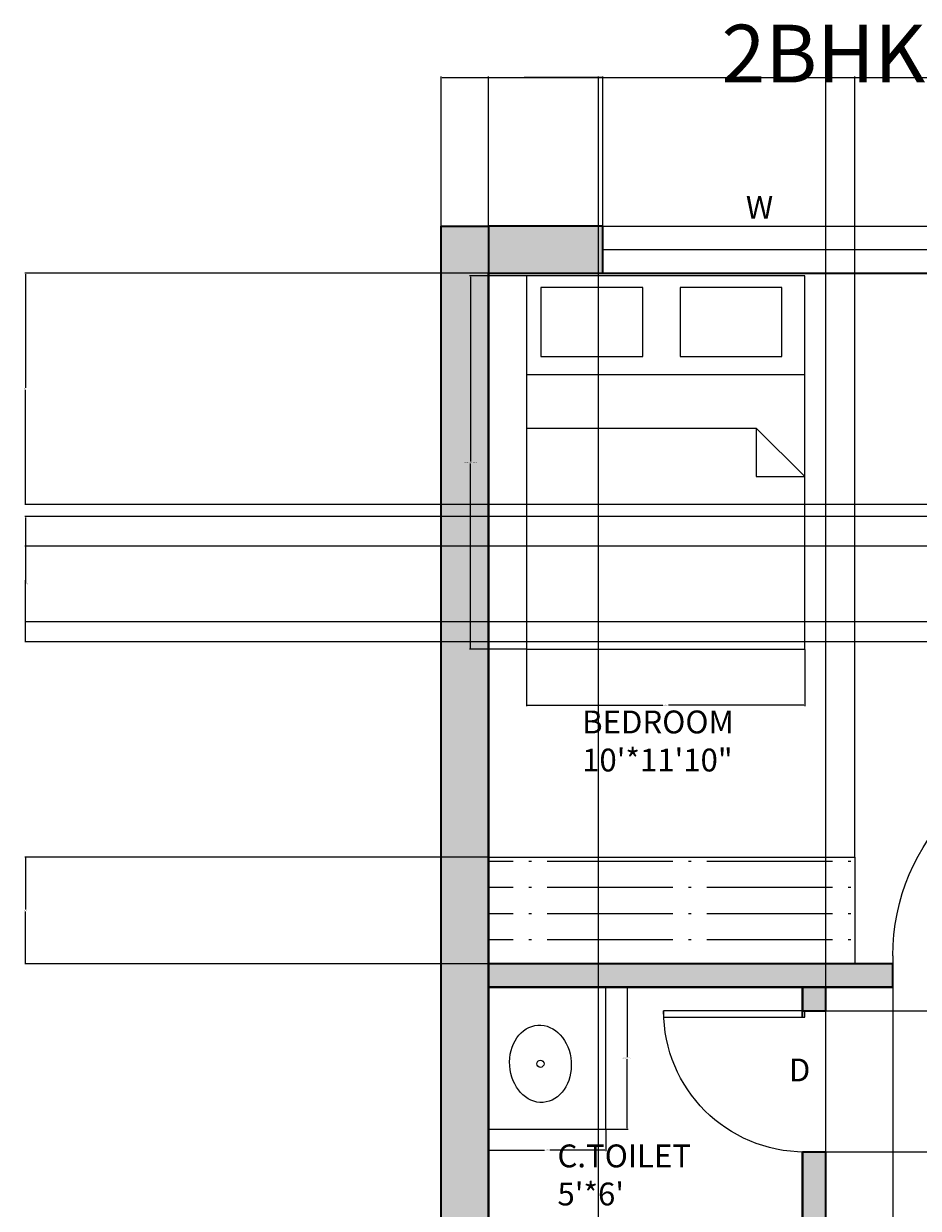
# Model space of a CAD drawing. Units: inches. Extents: x 2035 to 2384, y 1427 to 2020.
# Tile 5 of 7: x 2035 to 2206, y 1794 to 2020. Entities that reach past the tile are written whole.
import ezdxf

# ---------------------------------------------------------------- set-up
doc = ezdxf.new("R2010")
doc.units = ezdxf.units.IN
for name, color, linetype, lineweight in [('A-ANNO-DIMS', 2, 'Continuous', 18), ('A-ANNO-IDEN', 201, 'Continuous', 18), ('A-ANNO-TITL', 7, 'Continuous', 35), ('A-AREA-IDEN', 201, 'Continuous', 18), ('A-FLOR-CABN', 71, 'Continuous', 18), ('A-FLOR-CABN-PATT', 71, 'Continuous', 13), ('A-FLOR-FIXT', 9, 'Continuous', 18), ('A-WALL-PATT', 140, 'Continuous', 13), ('C-PROP', 7, 'Continuous', 25), ('DOOR', 52, 'Continuous', 25), ('FUR', 71, 'Continuous', 18), ('WALL', 140, 'Continuous', 35), ('WIN', 230, 'Continuous', 18)]:
    doc.layers.add(name, color=color, linetype=linetype, lineweight=lineweight)
doc.styles.get("Standard").update_dxf_attribs({"font": 'arial.ttf'})
doc.dimstyles.get("Standard").update_dxf_attribs({"dimtxt": 0.18, "dimasz": 0.18, "dimexe": 0.18, "dimexo": 0.0625, "dimgap": 0.09, "dimtad": 0, "dimtih": 1, "dimtoh": 1, "dimdec": 4, "dimzin": 0, "dimdsep": 46, "dimtxsty": 'Standard', "dimcen": 0.09, "dimadec": 0, "dimazin": 0, "dimtfac": 1, "dimtdec": 4, "dimtofl": 0, "dimtmove": 0, "dimatfit": 3, "dimfxl": 1, "dimtolj": 1, "dimtzin": 0, "dimarcsym": 0})

# ---------------------------------------------------------------- blocks, each defined once
blk = doc.blocks.new('*U2')
for p, q in [((0, 0), (0, -6)), ((40, 0), (40, -6))]:
    blk.add_line(p, q)
blk.add_lwpolyline([(0, 0), (0, 40), (1.75, 40), (1.75, 0)], close=True)
blk.add_arc((0, 0), 40, 0, 90)
blk = doc.blocks.new('BED-DOUBLE')
for p, q in [((18.86, 0), (18.86, 53.15)), ((38.37, 53.15), (29.1, 43.9)), ((38.37, 43.9), (38.37, 53.15)), ((29.1, 0), (29.1, 43.9)), ((29.1, 43.9), (38.37, 43.9))]:
    blk.add_line(p, q)
for points in [[(0, 0), (71.34, 0), (71.34, 53.15), (0, 53.15)], [(2.2, 29.34), (15.42, 29.34), (15.42, 48.81), (2.2, 48.81)], [(2.2, 2.74), (15.42, 2.74), (15.42, 22.21), (2.2, 22.21)]]:
    blk.add_lwpolyline(points, close=True)
blk = doc.blocks.new('BASIN-VANITY')
blk.add_lwpolyline([(0, 0), (22.45, 0), (22.45, 27.1), (0, 27.1)], close=True)
blk.add_circle((9.95, 12.48), 0.683)
blk.add_ellipse((9.95, 12.48), major_axis=(-0.5, 7.38), ratio=0.795414)
blk = doc.blocks.new('WIN-BEDROOM')
blk.add_line((0, 4.5), (63.76, 4.5))
blk.add_lwpolyline([(0, 9), (63.76, 9), (63.76, 0), (0, 0)], close=True)
blk = doc.blocks.new('*D12')
at = {"layer": 'A-ANNO-DIMS', "color": 0, "lineweight": -2, "transparency": 16777216}
for p, q in [((2130.97, 1971.85), (2120.15, 1971.85)), ((2120.33, 1971.67), (2120.33, 1936.36)), ((2120.33, 1900.69), (2120.33, 1935.99)), ((2130.97, 1900.51), (2120.15, 1900.51))]:
    blk.add_line(p, q, dxfattribs=at)
at = {"layer": 'A-ANNO-DIMS', "color": 0, "lineweight": 100, "transparency": 16777216}
for points in [[(2120.3, 1971.67), (2120.36, 1971.67), (2120.33, 1971.85)], [(2120.3, 1900.69), (2120.36, 1900.69), (2120.33, 1900.51)]]:
    blk.add_solid(points, dxfattribs=at)
at = {"layer": 'Defpoints', "color": 0, "lineweight": 100, "transparency": 16777216}
for p in [(2131.03, 1971.85), (2120.33, 1900.51), (2131.03, 1900.51)]:
    blk.add_point(p, dxfattribs=at)
at = {"layer": 'A-ANNO-DIMS', "color": 0, "transparency": 16777216, "insert": (2120.33, 1936.18), "char_height": 0.18, "attachment_point": 5}
blk.add_mtext('\\A1;DOUBLE BED 71 TYP.', dxfattribs=at)
blk = doc.blocks.new('*D13')
at = {"layer": 'A-ANNO-DIMS', "color": 0, "lineweight": -2, "transparency": 16777216}
for p, q in [((2131.03, 1900.45), (2131.03, 1889.63)), ((2184.19, 1900.45), (2184.19, 1889.63)), ((2131.21, 1889.81), (2157.08, 1889.81)), ((2184.01, 1889.81), (2158.14, 1889.81))]:
    blk.add_line(p, q, dxfattribs=at)
at = {"layer": 'A-ANNO-DIMS', "color": 0, "lineweight": 100, "transparency": 16777216}
for points in [[(2131.21, 1889.84), (2131.21, 1889.78), (2131.03, 1889.81)], [(2184.01, 1889.84), (2184.01, 1889.78), (2184.19, 1889.81)]]:
    blk.add_solid(points, dxfattribs=at)
at = {"layer": 'Defpoints', "color": 0, "lineweight": 100, "transparency": 16777216}
for p in [(2131.03, 1900.51), (2184.19, 1900.51), (2184.19, 1889.81)]:
    blk.add_point(p, dxfattribs=at)
at = {"layer": 'A-ANNO-DIMS', "color": 0, "transparency": 16777216, "insert": (2157.61, 1889.81), "char_height": 0.18, "attachment_point": 5}
blk.add_mtext('\\A1;53 TYP.', dxfattribs=at)
blk = doc.blocks.new('*D18')
at = {"layer": 'A-ANNO-DIMS', "color": 0, "lineweight": -2, "transparency": 16777216}
for p, q in [((2146.26, 1835.88), (2150.44, 1835.88)), ((2150.26, 1835.7), (2150.26, 1822.51)), ((2150.26, 1808.96), (2150.26, 1822.15)), ((2146.26, 1808.78), (2150.44, 1808.78))]:
    blk.add_line(p, q, dxfattribs=at)
at = {"layer": 'A-ANNO-DIMS', "color": 0, "lineweight": 100, "transparency": 16777216}
for points in [[(2150.23, 1835.7), (2150.29, 1835.7), (2150.26, 1835.88)], [(2150.23, 1808.96), (2150.29, 1808.96), (2150.26, 1808.78)]]:
    blk.add_solid(points, dxfattribs=at)
at = {"layer": 'Defpoints', "color": 0, "lineweight": 100, "transparency": 16777216}
for p in [(2146.2, 1835.88), (2150.26, 1835.88), (2146.2, 1808.78)]:
    blk.add_point(p, dxfattribs=at)
at = {"layer": 'A-ANNO-DIMS', "color": 0, "transparency": 16777216, "insert": (2150.26, 1822.33), "char_height": 0.18, "attachment_point": 5}
blk.add_mtext('\\A1;VANITY 27 TYP.', dxfattribs=at)
blk = doc.blocks.new('*D19')
at = {"layer": 'A-ANNO-DIMS', "color": 0, "lineweight": -2, "transparency": 16777216}
for p, q in [((2123.75, 1808.72), (2123.75, 1804.54)), ((2146.2, 1808.72), (2146.2, 1804.54)), ((2123.93, 1804.72), (2134.45, 1804.72)), ((2146.02, 1804.72), (2135.51, 1804.72))]:
    blk.add_line(p, q, dxfattribs=at)
at = {"layer": 'A-ANNO-DIMS', "color": 0, "lineweight": 100, "transparency": 16777216}
for points in [[(2123.93, 1804.75), (2123.93, 1804.69), (2123.75, 1804.72)], [(2146.02, 1804.75), (2146.02, 1804.69), (2146.2, 1804.72)]]:
    blk.add_solid(points, dxfattribs=at)
at = {"layer": 'Defpoints', "color": 0, "lineweight": 100, "transparency": 16777216}
for p in [(2123.75, 1808.78), (2146.2, 1808.78), (2146.2, 1804.72)]:
    blk.add_point(p, dxfattribs=at)
at = {"layer": 'A-ANNO-DIMS', "color": 0, "transparency": 16777216, "insert": (2134.98, 1804.72), "char_height": 0.18, "attachment_point": 5}
blk.add_mtext('\\A1;22 TYP.', dxfattribs=at)
blk = doc.blocks.new('*D22')
at = {"layer": 'A-ANNO-DIMS', "color": 0, "lineweight": -2, "transparency": 16777216}
for p, q in [((2114.75, 1981.44), (2114.75, 2009.96)), ((2114.93, 2009.78), (2234.46, 2009.78)), ((2354.57, 2009.78), (2235.04, 2009.78)), ((2354.75, 1981.44), (2354.75, 2009.96))]:
    blk.add_line(p, q, dxfattribs=at)
at = {"layer": 'A-ANNO-DIMS', "color": 0, "lineweight": 100, "transparency": 16777216}
for points in [[(2114.93, 2009.81), (2114.93, 2009.75), (2114.75, 2009.78)], [(2354.57, 2009.81), (2354.57, 2009.75), (2354.75, 2009.78)]]:
    blk.add_solid(points, dxfattribs=at)
at = {"layer": 'Defpoints', "color": 0, "lineweight": 100, "transparency": 16777216}
for p in [(2354.75, 2009.78), (2114.75, 1981.38), (2354.75, 1981.38)]:
    blk.add_point(p, dxfattribs=at)
at = {"layer": 'A-ANNO-DIMS', "color": 0, "transparency": 16777216, "insert": (2234.75, 2009.78), "char_height": 0.18, "attachment_point": 5}
blk.add_mtext('\\A1;240', dxfattribs=at)
blk = doc.blocks.new('*D33')
at = {"layer": 'A-ANNO-DIMS', "color": 0, "lineweight": -2, "transparency": 16777216}
for p, q in [((2114.75, 1981.44), (2114.75, 2009.96)), ((2114.93, 2009.78), (2129.79, 2009.78)), ((2145.44, 2009.78), (2130.58, 2009.78)), ((2145.62, 1981.44), (2145.62, 2009.96))]:
    blk.add_line(p, q, dxfattribs=at)
at = {"layer": 'A-ANNO-DIMS', "color": 0, "lineweight": 100, "transparency": 16777216}
for points in [[(2114.93, 2009.81), (2114.93, 2009.75), (2114.75, 2009.78)], [(2145.44, 2009.81), (2145.44, 2009.75), (2145.62, 2009.78)]]:
    blk.add_solid(points, dxfattribs=at)
at = {"layer": 'Defpoints', "color": 0, "lineweight": 100, "transparency": 16777216}
for p in [(2145.62, 2009.78), (2114.75, 1981.38), (2145.62, 1981.38)]:
    blk.add_point(p, dxfattribs=at)
at = {"layer": 'A-ANNO-DIMS', "color": 0, "transparency": 16777216, "insert": (2130.19, 2009.78), "char_height": 0.18, "attachment_point": 5}
blk.add_mtext('\\A1;30.87', dxfattribs=at)
blk = doc.blocks.new('*D38')
at = {"layer": 'A-ANNO-DIMS', "color": 0, "lineweight": -2, "transparency": 16777216}
for p, q in [((2183.82, 1831.37), (2383.33, 1831.37)), ((2383.15, 1831.19), (2383.15, 1818.07)), ((2383.15, 1804.58), (2383.15, 1817.7)), ((2183.82, 1804.4), (2383.33, 1804.4))]:
    blk.add_line(p, q, dxfattribs=at)
at = {"layer": 'A-ANNO-DIMS', "color": 0, "lineweight": 100, "transparency": 16777216}
for points in [[(2383.12, 1831.19), (2383.18, 1831.19), (2383.15, 1831.37)], [(2383.12, 1804.58), (2383.18, 1804.58), (2383.15, 1804.4)]]:
    blk.add_solid(points, dxfattribs=at)
at = {"layer": 'Defpoints', "color": 0, "lineweight": 100, "transparency": 16777216}
for p in [(2183.75, 1831.37), (2383.15, 1831.37), (2183.75, 1804.4)]:
    blk.add_point(p, dxfattribs=at)
at = {"layer": 'A-ANNO-DIMS', "color": 0, "transparency": 16777216, "insert": (2383.15, 1817.88), "char_height": 0.18, "attachment_point": 5}
blk.add_mtext('\\A1;26.97', dxfattribs=at)
blk = doc.blocks.new('*D40')
at = {"layer": 'A-ANNO-DIMS', "color": 0, "lineweight": -2, "transparency": 16777216}
for p, q in [((2201.01, 1835.82), (2201.01, 1427.17)), ((2241.01, 1835.82), (2241.01, 1427.17)), ((2201.19, 1427.35), (2220.79, 1427.35)), ((2240.83, 1427.35), (2221.24, 1427.35))]:
    blk.add_line(p, q, dxfattribs=at)
at = {"layer": 'A-ANNO-DIMS', "color": 0, "lineweight": 100, "transparency": 16777216}
for points in [[(2201.19, 1427.38), (2201.19, 1427.32), (2201.01, 1427.35)], [(2240.83, 1427.38), (2240.83, 1427.32), (2241.01, 1427.35)]]:
    blk.add_solid(points, dxfattribs=at)
at = {"layer": 'Defpoints', "color": 0, "lineweight": 100, "transparency": 16777216}
for p in [(2201.01, 1835.88), (2241.01, 1835.88), (2241.01, 1427.35)]:
    blk.add_point(p, dxfattribs=at)
at = {"layer": 'A-ANNO-DIMS', "color": 0, "transparency": 16777216, "insert": (2221.01, 1427.35), "char_height": 0.18, "attachment_point": 5}
blk.add_mtext('\\A1;40', dxfattribs=at)
blk = doc.blocks.new('*D43')
at = {"layer": 'A-ANNO-DIMS', "color": 0, "lineweight": -2, "transparency": 16777216}
for p, q in [((2243.69, 1972.38), (2035.17, 1972.38)), ((2035.35, 1972.2), (2035.35, 1950.44)), ((2035.35, 1928.31), (2035.35, 1950.07)), ((2243.69, 1928.13), (2035.17, 1928.13))]:
    blk.add_line(p, q, dxfattribs=at)
at = {"layer": 'A-ANNO-DIMS', "color": 0, "lineweight": 100, "transparency": 16777216}
for points in [[(2035.32, 1972.2), (2035.38, 1972.2), (2035.35, 1972.38)], [(2035.32, 1928.31), (2035.38, 1928.31), (2035.35, 1928.13)]]:
    blk.add_solid(points, dxfattribs=at)
at = {"layer": 'Defpoints', "color": 0, "lineweight": 100, "transparency": 16777216}
for p in [(2035.35, 1972.38), (2243.75, 1972.38), (2243.75, 1928.13)]:
    blk.add_point(p, dxfattribs=at)
at = {"layer": 'A-ANNO-DIMS', "color": 0, "transparency": 16777216, "insert": (2035.35, 1950.26), "char_height": 0.18, "attachment_point": 5}
blk.add_mtext('\\A1;44.25', dxfattribs=at)
blk = doc.blocks.new('*D44')
at = {"layer": 'A-ANNO-DIMS', "color": 0, "lineweight": -2, "transparency": 16777216}
for p, q in [((2284.64, 1925.88), (2035.17, 1925.88)), ((2035.35, 1925.7), (2035.35, 1914.06)), ((2035.35, 1902.06), (2035.35, 1913.7)), ((2284.64, 1901.88), (2035.17, 1901.88))]:
    blk.add_line(p, q, dxfattribs=at)
at = {"layer": 'A-ANNO-DIMS', "color": 0, "lineweight": 100, "transparency": 16777216}
for points in [[(2035.32, 1925.7), (2035.38, 1925.7), (2035.35, 1925.88)], [(2035.32, 1902.06), (2035.38, 1902.06), (2035.35, 1901.88)]]:
    blk.add_solid(points, dxfattribs=at)
at = {"layer": 'Defpoints', "color": 0, "lineweight": 100, "transparency": 16777216}
for p in [(2284.7, 1925.88), (2035.35, 1901.88), (2284.7, 1901.88)]:
    blk.add_point(p, dxfattribs=at)
at = {"layer": 'A-ANNO-DIMS', "color": 0, "transparency": 16777216, "insert": (2035.35, 1913.88), "char_height": 0.18, "attachment_point": 5}
blk.add_mtext('\\A1;24', dxfattribs=at)
blk = doc.blocks.new('*D47')
at = {"layer": 'A-ANNO-DIMS', "color": 0, "lineweight": -2, "transparency": 16777216}
for p, q in [((2288.13, 1920.21), (2035.17, 1920.21)), ((2035.35, 1920.03), (2035.35, 1913.16)), ((2035.35, 1905.93), (2035.35, 1912.8)), ((2288.13, 1905.75), (2035.17, 1905.75))]:
    blk.add_line(p, q, dxfattribs=at)
at = {"layer": 'A-ANNO-DIMS', "color": 0, "lineweight": 100, "transparency": 16777216}
for points in [[(2035.32, 1920.03), (2035.38, 1920.03), (2035.35, 1920.21)], [(2035.32, 1905.93), (2035.38, 1905.93), (2035.35, 1905.75)]]:
    blk.add_solid(points, dxfattribs=at)
at = {"layer": 'Defpoints', "color": 0, "lineweight": 100, "transparency": 16777216}
for p in [(2035.35, 1920.21), (2288.19, 1920.21), (2288.19, 1905.75)]:
    blk.add_point(p, dxfattribs=at)
at = {"layer": 'A-ANNO-DIMS', "color": 0, "transparency": 16777216, "insert": (2035.35, 1912.98), "char_height": 0.18, "attachment_point": 5}
blk.add_mtext('\\A1;14.463', dxfattribs=at)
blk = doc.blocks.new('*D60')
at = {"layer": 'A-ANNO-DIMS', "color": 0, "lineweight": -2, "transparency": 16777216}
for p, q in [((2193.76, 1860.83), (2193.76, 2009.96)), ((2193.94, 2009.78), (2218.54, 2009.78)), ((2243.57, 2009.78), (2218.97, 2009.78)), ((2243.75, 1840.44), (2243.75, 2009.96))]:
    blk.add_line(p, q, dxfattribs=at)
at = {"layer": 'A-ANNO-DIMS', "color": 0, "lineweight": 100, "transparency": 16777216}
for points in [[(2193.94, 2009.81), (2193.94, 2009.75), (2193.76, 2009.78)], [(2243.57, 2009.81), (2243.57, 2009.75), (2243.75, 2009.78)]]:
    blk.add_solid(points, dxfattribs=at)
at = {"layer": 'Defpoints', "color": 0, "lineweight": 100, "transparency": 16777216}
for p in [(2243.75, 2009.78), (2193.76, 1860.77), (2243.75, 1840.38)]:
    blk.add_point(p, dxfattribs=at)
at = {"layer": 'A-ANNO-DIMS', "color": 0, "transparency": 16777216, "insert": (2218.75, 2009.78), "char_height": 0.18, "attachment_point": 5}
blk.add_mtext('\\A1;50', dxfattribs=at)
blk = doc.blocks.new('*D61')
at = {"layer": 'A-ANNO-DIMS', "color": 0, "lineweight": -2, "transparency": 16777216}
for p, q in [((2123.69, 1860.77), (2035.17, 1860.77)), ((2035.35, 1860.59), (2035.35, 1850.76)), ((2035.35, 1840.56), (2035.35, 1850.39)), ((2123.69, 1840.38), (2035.17, 1840.38))]:
    blk.add_line(p, q, dxfattribs=at)
at = {"layer": 'A-ANNO-DIMS', "color": 0, "lineweight": 100, "transparency": 16777216}
for points in [[(2035.32, 1860.59), (2035.38, 1860.59), (2035.35, 1860.77)], [(2035.32, 1840.56), (2035.38, 1840.56), (2035.35, 1840.38)]]:
    blk.add_solid(points, dxfattribs=at)
at = {"layer": 'Defpoints', "color": 0, "lineweight": 100, "transparency": 16777216}
for p in [(2035.35, 1860.77), (2123.75, 1860.77), (2123.75, 1840.38)]:
    blk.add_point(p, dxfattribs=at)
at = {"layer": 'A-ANNO-DIMS', "color": 0, "transparency": 16777216, "insert": (2035.35, 1850.58), "char_height": 0.18, "attachment_point": 5}
blk.add_mtext('\\A1;20.39', dxfattribs=at)
blk = doc.blocks.new('*D62')
at = {"layer": 'A-ANNO-DIMS', "color": 0, "lineweight": -2, "transparency": 16777216}
for p, q in [((2123.75, 1624.27), (2123.75, 2009.96)), ((2123.93, 2009.78), (2133.8, 2009.78)), ((2144.6, 2009.78), (2134.73, 2009.78)), ((2144.78, 1624.27), (2144.78, 2009.96))]:
    blk.add_line(p, q, dxfattribs=at)
at = {"layer": 'A-ANNO-DIMS', "color": 0, "lineweight": 100, "transparency": 16777216}
for points in [[(2123.93, 2009.81), (2123.93, 2009.75), (2123.75, 2009.78)], [(2144.6, 2009.81), (2144.6, 2009.75), (2144.78, 2009.78)]]:
    blk.add_solid(points, dxfattribs=at)
at = {"layer": 'Defpoints', "color": 0, "lineweight": 100, "transparency": 16777216}
for p in [(2144.78, 2009.78), (2123.75, 1624.2), (2144.78, 1624.2)]:
    blk.add_point(p, dxfattribs=at)
at = {"layer": 'A-ANNO-DIMS', "color": 0, "transparency": 16777216, "insert": (2134.27, 2009.78), "char_height": 0.18, "attachment_point": 5}
blk.add_mtext('\\A1;21.028', dxfattribs=at)
blk = doc.blocks.new('*D70')
at = {"layer": 'A-ANNO-DIMS', "color": 0, "lineweight": -2, "transparency": 16777216}
for p, q in [((2188.25, 1804.46), (2188.25, 2009.96)), ((2188.43, 2009.78), (2213.67, 2009.78)), ((2239.7, 2009.78), (2214.46, 2009.78)), ((2239.88, 1811.3), (2239.88, 2009.96))]:
    blk.add_line(p, q, dxfattribs=at)
at = {"layer": 'A-ANNO-DIMS', "color": 0, "lineweight": 100, "transparency": 16777216}
for points in [[(2188.43, 2009.81), (2188.43, 2009.75), (2188.25, 2009.78)], [(2239.7, 2009.81), (2239.7, 2009.75), (2239.88, 2009.78)]]:
    blk.add_solid(points, dxfattribs=at)
at = {"layer": 'Defpoints', "color": 0, "lineweight": 100, "transparency": 16777216}
for p in [(2239.88, 2009.78), (2239.88, 1811.24), (2188.25, 1804.39)]:
    blk.add_point(p, dxfattribs=at)
at = {"layer": 'A-ANNO-DIMS', "color": 0, "transparency": 16777216, "insert": (2214.07, 2009.78), "char_height": 0.18, "attachment_point": 5}
blk.add_mtext('\\A1;51.62', dxfattribs=at)

msp = doc.modelspace()

# ---------------------------------------------------------------- hatches: boundary and pattern name
at = {"layer": 'A-FLOR-CABN-PATT'}
h = msp.add_hatch(dxfattribs=at)
h.set_pattern_fill('ACAD_ISO04W100', color=256)
h.paths.add_polyline_path([(2193.7559, 1860.7719), (2123.7529, 1860.7719), (2123.7529, 1840.3816), (2193.7559, 1840.3816)])
at = {"layer": 'A-WALL-PATT'}
h = msp.add_hatch(color=256, dxfattribs=at)
h.dxf.hatch_style = 1
h.paths.add_polyline_path([(2145.6215, 1981.3816), (2123.7529, 1981.3816), (2123.7529, 1972.3816), (2145.6215, 1972.3816)])
h.paths.add_polyline_path([(2354.7529, 1981.3816), (2209.3767, 1981.3816), (2209.3767, 1972.3816), (2354.7529, 1972.3816)])
h.paths.add_polyline_path([(2123.7529, 1981.3816), (2114.7529, 1981.3816), (2114.7529, 1505.8816), (2123.7529, 1505.8816)])
h.paths.add_polyline_path([(2248.2529, 1928.1316), (2243.7529, 1928.1316), (2243.7529, 1840.3816), (2248.2529, 1840.3816)])
h.paths.add_polyline_path([(2297.0514, 1930.3816), (2284.6994, 1930.3816), (2284.6994, 1925.8816), (2297.0514, 1925.8816)])
h.paths.add_polyline_path([(2345.7529, 1930.3816), (2333.1098, 1930.3816), (2333.1098, 1925.8816), (2345.7529, 1925.8816)])
h.paths.add_polyline_path([(2354.7529, 1972.3816), (2345.7529, 1972.3816), (2345.7529, 1501.3816), (2354.7529, 1501.3816)])
h.paths.add_polyline_path([(2188.2529, 1835.8816), (2183.7529, 1835.8816), (2183.7529, 1831.3677), (2184.207, 1831.3677), (2188.2529, 1831.3677)])
h.paths.add_polyline_path([(2188.2529, 1804.3949), (2184.207, 1804.3949), (2183.7529, 1804.3949), (2183.7529, 1685.3816), (2188.2529, 1685.3816)])
h.paths.add_polyline_path([(2273.5087, 1840.3816), (2241.0146, 1840.3816), (2241.0146, 1835.8816), (2273.5087, 1835.8816)])
h.paths.add_polyline_path([(2345.7529, 1840.3816), (2310.4577, 1840.3816), (2310.4577, 1835.8816), (2345.7529, 1835.8816)])
h.paths.add_polyline_path([(2161.9064, 1524.4315), (2196.2972, 1524.4315), (2196.2972, 1533.4306), (2161.9064, 1533.4306)], flags=9)
h.paths.add_polyline_path([(2279.3058, 1589.7515), (2308.9483, 1589.7515), (2308.9483, 1598.7506), (2279.3058, 1598.7506)], flags=9)
h.paths.add_polyline_path([(2242.9684, 1662.1655), (2279.0513, 1662.1655), (2279.0513, 1671.1647), (2242.9684, 1671.1647)], flags=9)
h.paths.add_polyline_path([(2154.6483, 1622.8242), (2195.1309, 1622.8242), (2195.1309, 1639.1195), (2154.6483, 1639.1195)], flags=9)
h.paths.add_polyline_path([(2138.8708, 1715.378), (2162.5199, 1715.378), (2162.5199, 1731.6734), (2138.8708, 1731.6734)], flags=9)
h.paths.add_polyline_path([(2135.5598, 1791.707), (2165.1993, 1791.707), (2165.1993, 1808.0024), (2135.5598, 1808.0024)], flags=9)
h.paths.add_polyline_path([(2245.1071, 1740.4502), (2279.0303, 1740.4502), (2279.0303, 1756.7455), (2245.1071, 1756.7455)], flags=9)
h.paths.add_polyline_path([(2284.7312, 1866.5552), (2313.6916, 1866.5552), (2313.6916, 1890.2034), (2284.7312, 1890.2034)], flags=9)
h.paths.add_polyline_path([(2139.9071, 1874.6496), (2173.8303, 1874.6496), (2173.8303, 1890.9449), (2139.9071, 1890.9449)], flags=9)
h = msp.add_hatch(color=256, dxfattribs=at)
h.dxf.hatch_style = 1
h.paths.add_polyline_path([(2236.7529, 1556.8816), (2209.3767, 1556.8816), (2209.3767, 1547.8816), (2236.7529, 1547.8816)])
h.paths.add_polyline_path([(2241.2529, 1680.8816), (2236.7529, 1680.8816), (2236.7529, 1547.8816), (2241.2529, 1547.8816)])
h.paths.add_polyline_path([(2241.2529, 1505.8816), (2114.7529, 1505.8816), (2114.7529, 1501.3816), (2241.2529, 1501.3816)])
h.paths.add_polyline_path([(2242.179, 1683.1823), (2242.179, 1685.3816), (2234.769, 1685.3816), (2234.769, 1680.8816), (2242.179, 1680.8816)])
h.paths.add_polyline_path([(2286.8795, 1685.3816), (2272.8549, 1685.3816), (2272.8549, 1683.1823), (2272.8549, 1680.8816), (2286.8795, 1680.8816)])
h.paths.add_polyline_path([(2345.7529, 1685.3816), (2329.513, 1685.3816), (2329.513, 1680.8816), (2345.7529, 1680.8816)])
h.paths.add_polyline_path([(2279.3058, 1589.7515), (2308.9483, 1589.7515), (2308.9483, 1598.7506), (2279.3058, 1598.7506)], flags=9)
h.paths.add_polyline_path([(2242.9684, 1662.1655), (2279.0513, 1662.1655), (2279.0513, 1671.1647), (2242.9684, 1671.1647)], flags=9)
h.paths.add_polyline_path([(2154.6483, 1622.8242), (2195.1309, 1622.8242), (2195.1309, 1639.1195), (2154.6483, 1639.1195)], flags=9)
h.paths.add_polyline_path([(2138.8708, 1715.378), (2162.5199, 1715.378), (2162.5199, 1731.6734), (2138.8708, 1731.6734)], flags=9)
h.paths.add_polyline_path([(2135.5598, 1791.707), (2165.1993, 1791.707), (2165.1993, 1808.0024), (2135.5598, 1808.0024)], flags=9)
h.paths.add_polyline_path([(2245.1071, 1740.4502), (2279.0303, 1740.4502), (2279.0303, 1756.7455), (2245.1071, 1756.7455)], flags=9)
h.paths.add_polyline_path([(2284.7312, 1866.5552), (2313.6916, 1866.5552), (2313.6916, 1890.2034), (2284.7312, 1890.2034)], flags=9)
h.paths.add_polyline_path([(2284.6985, 1943.1527), (2309.7208, 1943.1527), (2309.7208, 1959.448), (2284.6985, 1959.448)], flags=9)
h.paths.add_polyline_path([(2139.9071, 1874.6496), (2173.8303, 1874.6496), (2173.8303, 1890.9449), (2139.9071, 1890.9449)], flags=9)
h = msp.add_hatch(color=256, dxfattribs=at)
h.dxf.hatch_style = 1
h.paths.add_polyline_path([(2201.0146, 1840.3816), (2123.7529, 1840.3816), (2123.7529, 1835.8816), (2201.0146, 1835.8816)])
h.paths.add_polyline_path([(2136.2543, 1763.8816), (2123.7529, 1763.8816), (2123.7529, 1759.3816), (2136.2543, 1759.3816)])
h.paths.add_polyline_path([(2183.7529, 1763.8816), (2169.7769, 1763.8816), (2169.7769, 1759.3816), (2183.7529, 1759.3816)])
h.paths.add_polyline_path([(2152.8338, 1685.1369), (2152.8338, 1685.3816), (2123.7529, 1685.3816), (2123.7529, 1680.8816), (2152.8338, 1680.8816)])
h.paths.add_polyline_path([(2194.769, 1685.3816), (2181.2028, 1685.3816), (2181.2028, 1685.1369), (2181.2028, 1680.8816), (2194.769, 1680.8816)])
h.paths.add_polyline_path([(2145.6215, 1556.8816), (2123.7529, 1556.8816), (2123.7529, 1547.8816), (2145.6215, 1547.8816)])
h.paths.add_polyline_path([(2161.9064, 1524.4315), (2196.2972, 1524.4315), (2196.2972, 1533.4306), (2161.9064, 1533.4306)], flags=9)
h.paths.add_polyline_path([(2279.3058, 1589.7515), (2308.9483, 1589.7515), (2308.9483, 1598.7506), (2279.3058, 1598.7506)], flags=9)
h.paths.add_polyline_path([(2242.9684, 1662.1655), (2279.0513, 1662.1655), (2279.0513, 1671.1647), (2242.9684, 1671.1647)], flags=9)
h.paths.add_polyline_path([(2154.6483, 1622.8242), (2195.1309, 1622.8242), (2195.1309, 1639.1195), (2154.6483, 1639.1195)], flags=9)
h.paths.add_polyline_path([(2138.8708, 1715.378), (2162.5199, 1715.378), (2162.5199, 1731.6734), (2138.8708, 1731.6734)], flags=9)
h.paths.add_polyline_path([(2135.5598, 1791.707), (2165.1993, 1791.707), (2165.1993, 1808.0024), (2135.5598, 1808.0024)], flags=9)
h.paths.add_polyline_path([(2245.1071, 1740.4502), (2279.0303, 1740.4502), (2279.0303, 1756.7455), (2245.1071, 1756.7455)], flags=9)
h.paths.add_polyline_path([(2284.7312, 1866.5552), (2313.6916, 1866.5552), (2313.6916, 1890.2034), (2284.7312, 1890.2034)], flags=9)
h.paths.add_polyline_path([(2284.6985, 1943.1527), (2309.7208, 1943.1527), (2309.7208, 1959.448), (2284.6985, 1959.448)], flags=9)
h.paths.add_polyline_path([(2139.9071, 1874.6496), (2173.8303, 1874.6496), (2173.8303, 1890.9449), (2139.9071, 1890.9449)], flags=9)

# ---------------------------------------------------------------- linework, layer by layer
at = {"layer": 'A-FLOR-CABN'}
msp.add_lwpolyline([(2193.7559, 1840.3816), (2123.7529, 1840.3816), (2123.7529, 1860.7719), (2193.7559, 1860.7719)], close=True, dxfattribs=at)
at = {"layer": 'C-PROP'}
for p, q in [((2114.7529, 1981.3816), (2354.7529, 1981.3816)), ((2114.7529, 1501.3816), (2114.7529, 1981.3816))]:
    msp.add_line(p, q, dxfattribs=at)
msp.add_lwpolyline([(2114.7529, 1981.3816), (2354.7529, 1981.3816), (2354.7529, 1501.3816), (2114.7529, 1501.3816)], close=True, dxfattribs=at)
at = {"layer": 'WALL'}
for p, q in [((2123.7529, 1972.3816), (2243.7529, 1972.3816)), ((2201.0146, 1840.3816), (2123.7529, 1840.3816)), ((2123.7529, 1835.8816), (2123.7529, 1763.8816)), ((2201.0146, 1835.8816), (2123.7529, 1835.8816)), ((2183.7529, 1830.1877), (2183.7529, 1835.8816)), ((2188.2529, 1831.3677), (2188.2529, 1835.8816)), ((2183.7529, 1763.8816), (2183.7529, 1804.3987)), ((2188.2529, 1759.3816), (2188.2529, 1804.3949))]:
    msp.add_line(p, q, dxfattribs=at)
for points in [[(2114.7529, 1981.3816), (2123.7529, 1981.3816), (2123.7529, 1505.8816), (2114.7529, 1505.8816)], [(2145.6215, 1981.3816), (2123.7529, 1981.3816), (2123.7529, 1972.3816), (2145.6215, 1972.3816)], [(2123.7529, 1835.8816), (2201.0146, 1835.8816), (2201.0146, 1840.3816), (2123.7529, 1840.3816)], [(2183.7529, 1831.3677), (2188.2529, 1831.3677), (2188.2529, 1835.8816), (2183.7529, 1835.8816)], [(2188.2529, 1804.3949), (2183.7529, 1804.3949), (2183.7529, 1685.3816), (2188.2529, 1685.3816)]]:
    msp.add_lwpolyline(points, close=True, dxfattribs=at)
msp.add_lwpolyline([(2241.2529, 1552.3816), (2241.2529, 1505.8816), (2123.7529, 1505.8816), (2123.7529, 1972.3816), (2345.7529, 1972.3816), (2345.7529, 1503.6316), (2323.1125, 1503.6316)], dxfattribs=at)

# ---------------------------------------------------------------- block references
at = {"layer": 'A-FLOR-FIXT'}
msp.add_blockref('BASIN-VANITY', (2123.7529, 1808.7809), dxfattribs=at)
at = {"layer": 'DOOR', "xscale": -1}
msp.add_blockref('*U2', (2241.0146, 1841.8816), dxfattribs=at)
at = {"layer": 'DOOR', "xscale": -0.674321063966273, "yscale": 0.674321063966273, "zscale": 0.674321063966273, "rotation": 90}
msp.add_blockref('*U2', (2184.207, 1831.3677), dxfattribs=at)
at = {"layer": 'FUR', "rotation": 270.0000000000002}
msp.add_blockref('BED-DOUBLE', (2131.0338, 1971.8455), dxfattribs=at)
at = {"layer": 'WIN'}
msp.add_blockref('WIN-BEDROOM', (2145.6215, 1972.3816), dxfattribs=at)

# ---------------------------------------------------------------- texts
at = {"layer": 'A-ANNO-IDEN', "char_height": 4.367, "attachment_point": 1}
for s, insert in [('W', (2172.9384, 1987.15)), ('D', (2181.1657, 1822.2618))]:
    msp.add_mtext_dynamic_manual_height_columns(s, width=88.030619, gutter_width=21.835, heights=[0], dxfattribs=dict(at, insert=insert))
at = {"layer": 'A-ANNO-TITL', "insert": (2168.3128, 2019.8582), "char_height": 11.035976, "attachment_point": 1}
msp.add_mtext_dynamic_manual_height_columns('2BHK HOUSE PLAN', width=742.455452, gutter_width=55.1799, heights=[0], dxfattribs=at)
at = {"layer": 'A-AREA-IDEN', "char_height": 4.367, "attachment_point": 1}
for s, insert in [('BEDROOM\\P10\'*11\'10"', (2141.6631, 1888.7748)), ("C.TOILET\\P5'*6'", (2136.9553, 1805.8323))]:
    msp.add_mtext_dynamic_manual_height_columns(s, width=88.030619, gutter_width=21.835, heights=[0], dxfattribs=dict(at, insert=insert))

# ---------------------------------------------------------------- dimensions: what is measured, and where the dimension line sits
at = {"layer": 'A-ANNO-DIMS'}
for base, p1, p2, override, picture, middle in [((2354.7529, 2009.7816), (2114.7529, 1981.3816), (2354.7529, 1981.3816), {"dimdec": 0, "dimlfac": 1, "dimrnd": 0, "dimzin": 0, "dimdsep": 46, "dimlunit": 2}, '*D22', (2234.7529, 2009.7816)), ((2145.6215, 2009.7816), (2114.7529, 1981.3816), (2145.6215, 1981.3816), {"dimdec": 2, "dimlfac": 1, "dimrnd": 0, "dimzin": 0, "dimdsep": 46, "dimlunit": 2}, '*D33', (2130.1872, 2009.7816)), ((2144.7806, 2009.7816), (2123.7529, 1624.204), (2144.7806, 1624.204), {"dimdec": 3, "dimlfac": 1, "dimrnd": 0, "dimzin": 0, "dimdsep": 46, "dimlunit": 2}, '*D62', (2134.2668, 2009.7816)), ((2239.8773, 2009.7816), (2188.2529, 1804.3949), (2239.8773, 1811.2357), {"dimdec": 2, "dimlfac": 1, "dimrnd": 0, "dimzin": 0, "dimdsep": 46, "dimlunit": 2}, '*D70', (2214.0651, 2009.7816)), ((2243.7529, 2009.7816), (2193.7559, 1860.7719), (2243.7529, 1840.3816), {"dimdec": 0, "dimlfac": 1, "dimrnd": 0, "dimzin": 0, "dimdsep": 46, "dimlunit": 2}, '*D60', (2218.7544, 2009.7816)), ((2241.0146, 1427.3483), (2201.0146, 1835.8816), (2241.0146, 1835.8816), {"dimdec": 0, "dimlfac": 1, "dimrnd": 0, "dimzin": 0, "dimdsep": 46, "dimlunit": 2}, '*D40', (2221.0146, 1427.3483))]:
    dim = msp.add_linear_dim(base=base, p1=p1, p2=p2, dimstyle='Standard', override=override, dxfattribs=at)
    dim.commit()
    dim.dimension.update_dxf_attribs({"geometry": picture, "text_midpoint": middle})
for base, p1, p2, override, picture, middle in [((2035.3529, 1972.3816), (2243.7529, 1928.1316), (2243.7529, 1972.3816), {"dimdec": 2, "dimlfac": 1, "dimrnd": 0, "dimzin": 0, "dimdsep": 46, "dimlunit": 2}, '*D43', (2035.3529, 1950.2566)), ((2035.3529, 1901.8816), (2284.6994, 1925.8816), (2284.6994, 1901.8816), {"dimdec": 0, "dimlfac": 1, "dimrnd": 0, "dimzin": 0, "dimdsep": 46, "dimlunit": 2}, '*D44', (2035.3529, 1913.8816)), ((2035.3529, 1920.2089), (2288.1887, 1905.7459), (2288.1887, 1920.2089), {"dimdec": 3, "dimlfac": 1, "dimrnd": 0, "dimzin": 0, "dimdsep": 46, "dimlunit": 2}, '*D47', (2035.3529, 1912.9774)), ((2035.3529, 1860.7719), (2123.7529, 1840.3816), (2123.7529, 1860.7719), {"dimdec": 2, "dimlfac": 1, "dimrnd": 0, "dimzin": 0, "dimdsep": 46, "dimlunit": 2}, '*D61', (2035.3529, 1850.5767)), ((2383.1529, 1831.3677), (2183.7529, 1804.3987), (2183.7529, 1831.3677), {"dimdec": 2, "dimlfac": 1, "dimrnd": 0, "dimzin": 0, "dimdsep": 46, "dimlunit": 2}, '*D38', (2383.1529, 1817.8832))]:
    dim = msp.add_linear_dim(base=base, p1=p1, p2=p2, angle=90, dimstyle='Standard', override=override, dxfattribs=at)
    dim.commit()
    dim.dimension.update_dxf_attribs({"geometry": picture, "text_midpoint": middle})
for base, p1, p2, angle, text, picture, middle in [((2120.3334, 1900.5095), (2131.0338, 1971.8455), (2131.0338, 1900.5095), 270, 'DOUBLE BED <> TYP.', '*D12', (2120.3334, 1936.1775)), ((2184.1878, 1889.8091), (2131.0338, 1900.5095), (2184.1878, 1900.5095), 0, '<> TYP.', '*D13', (2157.6108, 1889.8091)), ((2150.2639, 1835.8816), (2146.1988, 1808.7809), (2146.1988, 1835.8816), 90, 'VANITY <> TYP.', '*D18', (2150.2639, 1822.3312))]:
    dim = msp.add_linear_dim(base=base, p1=p1, p2=p2, angle=angle, text=text, dimstyle='Standard', override={"dimdec": 0, "dimlfac": 1, "dimrnd": 0, "dimzin": 0, "dimdsep": 46, "dimlunit": 2}, dxfattribs=at)
    dim.commit()
    dim.dimension.update_dxf_attribs({"geometry": picture, "text_midpoint": middle})
dim = msp.add_linear_dim(base=(2146.1988, 1804.7158), p1=(2123.7529, 1808.7809), p2=(2146.1988, 1808.7809), text='<> TYP.', dimstyle='Standard', override={"dimdec": 0, "dimlfac": 1, "dimrnd": 0, "dimzin": 0, "dimdsep": 46, "dimlunit": 2}, dxfattribs=at)
dim.commit()
dim.dimension.update_dxf_attribs({"geometry": '*D19', "text_midpoint": (2134.9759, 1804.7158)})

doc.saveas('drawing.dxf')
